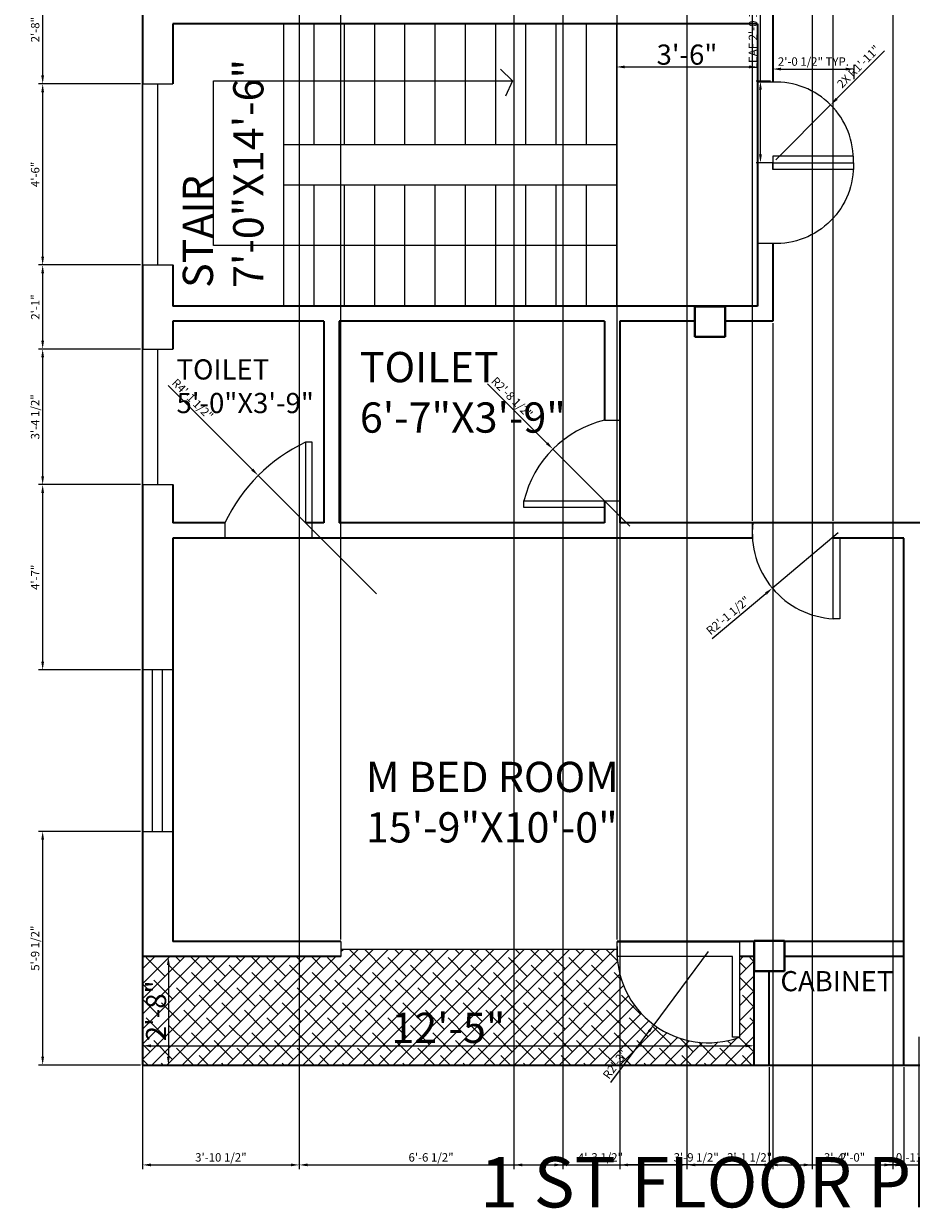
# Model space of a CAD drawing. Units: millimetres. Extents: x 2124 to 2653, y 1244 to 1836.
# Tile 1 of 4: x 2124 to 2389, y 1244 to 1597. Entities that reach past the tile are written whole.
import ezdxf

# ---------------------------------------------------------------- set-up
doc = ezdxf.new("R2010")
doc.units = ezdxf.units.MM
for name, color, linetype, lineweight in [('A-ANNO-DIMS', 2, 'Continuous', 18), ('A-ANNO-TEXT', 7, 'Continuous', 18), ('A-ANNO-TITL', 7, 'Continuous', 35), ('A-AREA-IDEN', 7, 'Continuous', 18), ('A-COLS', 1, 'Continuous', 40), ('A-DOOR', 3, 'Continuous', 18), ('A-FLOR-PATT', 252, 'Continuous', 13), ('A-FLOR-STRS', 32, 'Continuous', 18), ('A-GLAZ', 4, 'Continuous', 18), ('A-WALL', 7, 'Continuous', 35)]:
    doc.layers.add(name, color=color, linetype=linetype, lineweight=lineweight)
doc.styles.get("Standard").update_dxf_attribs({"font": 'arial.ttf'})
doc.dimstyles.new('ISO-25', dxfattribs={"dimtxt": 2.5, "dimasz": 2.5, "dimexe": 1.25, "dimexo": 0.625, "dimtad": 1, "dimdec": 0, "dimlunit": 3, "dimtxsty": 'Standard', "dimcen": 2.5, "dimadec": 0, "dimazin": 0, "dimtfac": 1, "dimtdec": 0, "dimtmove": 0, "dimatfit": 3, "dimfxl": 1, "dimarcsym": 0})

# ---------------------------------------------------------------- blocks, each defined once
blk = doc.blocks.new('*D1')
at = {"layer": 'A-ANNO-DIMS', "color": 0, "lineweight": -2, "transparency": 16777216}
for p, q in [((2300.76, 1596.12), (2300.76, 1582.64)), ((2342.76, 1596.12), (2342.76, 1582.64)), ((2303.26, 1583.89), (2340.26, 1583.89))]:
    blk.add_line(p, q, dxfattribs=at)
at = {"layer": 'A-ANNO-DIMS', "color": 0, "transparency": 16777216}
for points in [[(2303.26, 1584.31), (2303.26, 1583.47), (2300.76, 1583.89)], [(2340.26, 1584.31), (2340.26, 1583.47), (2342.76, 1583.89)]]:
    blk.add_solid(points, dxfattribs=at)
at = {"layer": 'Defpoints', "color": 0, "transparency": 16777216}
for p in [(2300.76, 1596.74), (2342.76, 1596.74), (2342.76, 1583.89)]:
    blk.add_point(p, dxfattribs=at)
at = {"layer": 'A-ANNO-DIMS', "color": 0, "transparency": 16777216, "insert": (2321.76, 1587.55), "char_height": 2.5, "width": 10.4079, "attachment_point": 5}
blk.add_mtext('{\\fCambria|b0|i0|c0|p18;\\H2.4x;3\'-6"}', dxfattribs=at)
blk = doc.blocks.new('*D5')
at = {"layer": 'A-ANNO-DIMS', "color": 0, "lineweight": -2, "transparency": 16777216}
for p, q in [((2160.38, 1319.24), (2168.7, 1319.24)), ((2167.45, 1316.74), (2167.45, 1289.47)), ((2160.38, 1286.97), (2168.7, 1286.97))]:
    blk.add_line(p, q, dxfattribs=at)
at = {"layer": 'A-ANNO-DIMS', "color": 0, "transparency": 16777216}
for points in [[(2167.04, 1316.74), (2167.87, 1316.74), (2167.45, 1319.24)], [(2167.04, 1289.47), (2167.87, 1289.47), (2167.45, 1286.97)]]:
    blk.add_solid(points, dxfattribs=at)
at = {"layer": 'Defpoints', "color": 0, "transparency": 16777216}
for p in [(2159.76, 1319.24), (2159.76, 1286.97), (2167.45, 1286.97)]:
    blk.add_point(p, dxfattribs=at)
at = {"layer": 'A-ANNO-DIMS', "color": 0, "transparency": 16777216, "insert": (2163.79, 1303.11), "char_height": 2.5, "attachment_point": 5, "rotation": 90}
blk.add_mtext('{\\fCambria|b0|i0|c0|p18;\\H2.4x;2\'-8"}', dxfattribs=at)
blk = doc.blocks.new('*D6')
at = {"layer": 'A-ANNO-DIMS', "color": 0, "lineweight": -2, "transparency": 16777216}
for p, q in [((2159.76, 1287.6), (2159.76, 1293.95)), ((2341.76, 1287.6), (2341.76, 1293.95)), ((2162.26, 1292.7), (2339.26, 1292.7))]:
    blk.add_line(p, q, dxfattribs=at)
at = {"layer": 'A-ANNO-DIMS', "color": 0, "transparency": 16777216}
for points in [[(2162.26, 1293.12), (2162.26, 1292.28), (2159.76, 1292.7)], [(2339.26, 1293.12), (2339.26, 1292.28), (2341.76, 1292.7)]]:
    blk.add_solid(points, dxfattribs=at)
at = {"layer": 'Defpoints', "color": 0, "transparency": 16777216}
for p in [(2341.76, 1292.7), (2159.76, 1286.97), (2341.76, 1286.97)]:
    blk.add_point(p, dxfattribs=at)
at = {"layer": 'A-ANNO-DIMS', "color": 0, "transparency": 16777216, "insert": (2250.76, 1298.04), "char_height": 2.5, "width": 30.6159, "attachment_point": 5}
blk.add_mtext('{\\fCambria|b0|i0|c0|p18;\\H3.6x;12\'-5"}', dxfattribs=at)
blk = doc.blocks.new('WINDOW-4FT')
for p, q in [((48, 9), (0, 9)), ((0, 9), (0, 0)), ((48, 0), (48, 9)), ((48, 6), (0, 6)), ((48, 3), (0, 3)), ((0, 0), (48, 0))]:
    blk.add_line(p, q)
blk = doc.blocks.new('COLUMN-9IN-SQ')
for p, q in [((9, 9), (0, 9)), ((0, 9), (0, 0)), ((9, 0), (9, 9)), ((0, 0), (9, 0))]:
    blk.add_line(p, q)
blk = doc.blocks.new('DOOR-2FT-STAIR-LEAF')
for p, q in [((0, 2), (0, 0)), ((24, 2), (0, 2)), ((24, 0), (24, 2)), ((0, 0), (24, 0))]:
    blk.add_line(p, q)
blk.add_arc((0.91, 0.91), 23.11, 357.7485, 92.2515)
blk = doc.blocks.new('*D20')
at = {"layer": 'A-ANNO-DIMS', "color": 0, "lineweight": -2, "transparency": 16777216}
for p, q in [((2343.62, 1579.62), (2343.62, 1614.03)), ((2346.63, 1579.62), (2342.37, 1579.62)), ((2343.62, 1557.86), (2343.62, 1577.12)), ((2346.63, 1555.36), (2342.37, 1555.36))]:
    blk.add_line(p, q, dxfattribs=at)
at = {"layer": 'A-ANNO-DIMS', "color": 0, "transparency": 16777216}
for points in [[(2343.2, 1577.12), (2344.04, 1577.12), (2343.62, 1579.62)], [(2343.2, 1557.86), (2344.04, 1557.86), (2343.62, 1555.36)]]:
    blk.add_solid(points, dxfattribs=at)
at = {"layer": 'Defpoints', "color": 0, "transparency": 16777216}
for p in [(2343.62, 1579.62), (2347.26, 1579.62), (2347.26, 1555.36)]:
    blk.add_point(p, dxfattribs=at)
at = {"layer": 'A-ANNO-DIMS', "color": 0, "transparency": 16777216, "insert": (2341.7, 1598.07), "char_height": 2.5, "attachment_point": 5, "rotation": 90}
blk.add_mtext('LEAF 2\'-0 1/2" TYP.', dxfattribs=at)
blk = doc.blocks.new('*D21')
at = {"layer": 'A-ANNO-DIMS', "color": 0, "lineweight": -2, "transparency": 16777216}
for p, q in [((2347.26, 1580.24), (2347.26, 1584.51)), ((2349.76, 1583.26), (2369.01, 1583.26)), ((2371.51, 1580.24), (2371.51, 1584.51))]:
    blk.add_line(p, q, dxfattribs=at)
at = {"layer": 'A-ANNO-DIMS', "color": 0, "transparency": 16777216}
for points in [[(2349.76, 1583.67), (2349.76, 1582.84), (2347.26, 1583.26)], [(2369.01, 1583.67), (2369.01, 1582.84), (2371.51, 1583.26)]]:
    blk.add_solid(points, dxfattribs=at)
at = {"layer": 'Defpoints', "color": 0, "transparency": 16777216}
for p in [(2371.51, 1583.26), (2347.26, 1579.62), (2371.51, 1579.62)]:
    blk.add_point(p, dxfattribs=at)
at = {"layer": 'A-ANNO-DIMS', "color": 0, "transparency": 16777216, "insert": (2359.38, 1585.17), "char_height": 2.5, "attachment_point": 5}
blk.add_mtext('2\'-0 1/2" TYP.', dxfattribs=at)
blk = doc.blocks.new('*D29')
at = {"layer": 'A-ANNO-DIMS', "color": 0, "lineweight": -2, "transparency": 16777216}
for p, q in [((2159.13, 1356.5), (2128.81, 1356.5)), ((2130.06, 1289.47), (2130.06, 1354)), ((2159.13, 1286.97), (2128.81, 1286.97))]:
    blk.add_line(p, q, dxfattribs=at)
at = {"layer": 'A-ANNO-DIMS', "color": 0, "transparency": 16777216}
for points in [[(2129.64, 1354), (2130.47, 1354), (2130.06, 1356.5)], [(2129.64, 1289.47), (2130.47, 1289.47), (2130.06, 1286.97)]]:
    blk.add_solid(points, dxfattribs=at)
at = {"layer": 'Defpoints', "color": 0, "transparency": 16777216}
for p in [(2130.06, 1356.5), (2159.76, 1356.5), (2159.76, 1286.97)]:
    blk.add_point(p, dxfattribs=at)
at = {"layer": 'A-ANNO-DIMS', "color": 0, "transparency": 16777216, "insert": (2128.14, 1321.74), "char_height": 2.5, "attachment_point": 5, "rotation": 90}
blk.add_mtext('5\'-9 1/2"', dxfattribs=at)
blk = doc.blocks.new('*D30')
at = {"layer": 'A-ANNO-DIMS', "color": 0, "lineweight": -2, "transparency": 16777216}
for p, q in [((2159.13, 1459.63), (2128.81, 1459.63)), ((2130.06, 1407), (2130.06, 1457.13)), ((2159.13, 1404.5), (2128.81, 1404.5))]:
    blk.add_line(p, q, dxfattribs=at)
at = {"layer": 'A-ANNO-DIMS', "color": 0, "transparency": 16777216}
for points in [[(2129.64, 1457.13), (2130.47, 1457.13), (2130.06, 1459.63)], [(2129.64, 1407), (2130.47, 1407), (2130.06, 1404.5)]]:
    blk.add_solid(points, dxfattribs=at)
at = {"layer": 'Defpoints', "color": 0, "transparency": 16777216}
for p in [(2130.06, 1459.63), (2159.76, 1459.63), (2159.76, 1404.5)]:
    blk.add_point(p, dxfattribs=at)
at = {"layer": 'A-ANNO-DIMS', "color": 0, "transparency": 16777216, "insert": (2128.18, 1432.07), "char_height": 2.5, "attachment_point": 5, "rotation": 90}
blk.add_mtext('4\'-7"', dxfattribs=at)
blk = doc.blocks.new('*D31')
at = {"layer": 'A-ANNO-DIMS', "color": 0, "lineweight": -2, "transparency": 16777216}
for p, q in [((2159.13, 1499.97), (2128.81, 1499.97)), ((2130.06, 1462.13), (2130.06, 1497.47)), ((2159.13, 1459.63), (2128.81, 1459.63))]:
    blk.add_line(p, q, dxfattribs=at)
at = {"layer": 'A-ANNO-DIMS', "color": 0, "transparency": 16777216}
for points in [[(2129.64, 1497.47), (2130.47, 1497.47), (2130.06, 1499.97)], [(2129.64, 1462.13), (2130.47, 1462.13), (2130.06, 1459.63)]]:
    blk.add_solid(points, dxfattribs=at)
at = {"layer": 'Defpoints', "color": 0, "transparency": 16777216}
for p in [(2130.06, 1499.97), (2159.76, 1499.97), (2159.76, 1459.63)]:
    blk.add_point(p, dxfattribs=at)
at = {"layer": 'A-ANNO-DIMS', "color": 0, "transparency": 16777216, "insert": (2128.14, 1479.8), "char_height": 2.5, "attachment_point": 5, "rotation": 90}
blk.add_mtext('3\'-4 1/2"', dxfattribs=at)
blk = doc.blocks.new('*D32')
at = {"layer": 'A-ANNO-DIMS', "color": 0, "lineweight": -2, "transparency": 16777216}
for p, q in [((2159.13, 1524.98), (2128.81, 1524.98)), ((2130.06, 1502.47), (2130.06, 1522.48)), ((2159.13, 1499.97), (2128.81, 1499.97))]:
    blk.add_line(p, q, dxfattribs=at)
at = {"layer": 'A-ANNO-DIMS', "color": 0, "transparency": 16777216}
for points in [[(2129.64, 1522.48), (2130.47, 1522.48), (2130.06, 1524.98)], [(2129.64, 1502.47), (2130.47, 1502.47), (2130.06, 1499.97)]]:
    blk.add_solid(points, dxfattribs=at)
at = {"layer": 'Defpoints', "color": 0, "transparency": 16777216}
for p in [(2130.06, 1524.98), (2159.76, 1524.98), (2159.76, 1499.97)]:
    blk.add_point(p, dxfattribs=at)
at = {"layer": 'A-ANNO-DIMS', "color": 0, "transparency": 16777216, "insert": (2128.18, 1512.47), "char_height": 2.5, "attachment_point": 5, "rotation": 90}
blk.add_mtext('2\'-1"', dxfattribs=at)
blk = doc.blocks.new('*D33')
at = {"layer": 'A-ANNO-DIMS', "color": 0, "lineweight": -2, "transparency": 16777216}
for p, q in [((2159.13, 1578.86), (2128.81, 1578.86)), ((2130.06, 1527.48), (2130.06, 1576.36)), ((2159.13, 1524.98), (2128.81, 1524.98))]:
    blk.add_line(p, q, dxfattribs=at)
at = {"layer": 'A-ANNO-DIMS', "color": 0, "transparency": 16777216}
for points in [[(2129.64, 1576.36), (2130.47, 1576.36), (2130.06, 1578.86)], [(2129.64, 1527.48), (2130.47, 1527.48), (2130.06, 1524.98)]]:
    blk.add_solid(points, dxfattribs=at)
at = {"layer": 'Defpoints', "color": 0, "transparency": 16777216}
for p in [(2130.06, 1578.86), (2159.76, 1578.86), (2159.76, 1524.98)]:
    blk.add_point(p, dxfattribs=at)
at = {"layer": 'A-ANNO-DIMS', "color": 0, "transparency": 16777216, "insert": (2128.15, 1551.92), "char_height": 2.5, "attachment_point": 5, "rotation": 90}
blk.add_mtext('4\'-6"', dxfattribs=at)
blk = doc.blocks.new('*D34')
at = {"layer": 'A-ANNO-DIMS', "color": 0, "lineweight": -2, "transparency": 16777216}
for p, q in [((2159.13, 1611.09), (2128.81, 1611.09)), ((2130.06, 1581.36), (2130.06, 1608.59)), ((2159.13, 1578.86), (2128.81, 1578.86))]:
    blk.add_line(p, q, dxfattribs=at)
at = {"layer": 'A-ANNO-DIMS', "color": 0, "transparency": 16777216}
for points in [[(2129.64, 1608.59), (2130.47, 1608.59), (2130.06, 1611.09)], [(2129.64, 1581.36), (2130.47, 1581.36), (2130.06, 1578.86)]]:
    blk.add_solid(points, dxfattribs=at)
at = {"layer": 'Defpoints', "color": 0, "transparency": 16777216}
for p in [(2130.06, 1611.09), (2159.76, 1611.09), (2159.76, 1578.86)]:
    blk.add_point(p, dxfattribs=at)
at = {"layer": 'A-ANNO-DIMS', "color": 0, "transparency": 16777216, "insert": (2128.15, 1594.98), "char_height": 2.5, "attachment_point": 5, "rotation": 90}
blk.add_mtext('2\'-8"', dxfattribs=at)
blk = doc.blocks.new('*D36')
at = {"layer": 'A-ANNO-DIMS', "color": 0, "lineweight": -2, "transparency": 16777216}
for p, q in [((2159.76, 1753.12), (2159.76, 1256.02)), ((2206.41, 1748.62), (2206.41, 1256.02)), ((2162.26, 1257.27), (2203.91, 1257.27))]:
    blk.add_line(p, q, dxfattribs=at)
at = {"layer": 'A-ANNO-DIMS', "color": 0, "transparency": 16777216}
for points in [[(2162.26, 1257.69), (2162.26, 1256.86), (2159.76, 1257.27)], [(2203.91, 1257.69), (2203.91, 1256.86), (2206.41, 1257.27)]]:
    blk.add_solid(points, dxfattribs=at)
at = {"layer": 'Defpoints', "color": 0, "transparency": 16777216}
for p in [(2159.76, 1753.74), (2206.41, 1749.24), (2206.41, 1257.27)]:
    blk.add_point(p, dxfattribs=at)
at = {"layer": 'A-ANNO-DIMS', "color": 0, "transparency": 16777216, "insert": (2183.08, 1259.19), "char_height": 2.5, "attachment_point": 5}
blk.add_mtext('3\'-10 1/2"', dxfattribs=at)
blk = doc.blocks.new('*D37')
at = {"layer": 'A-ANNO-DIMS', "color": 0, "lineweight": -2, "transparency": 16777216}
for p, q in [((2206.41, 1748.62), (2206.41, 1256.02)), ((2284.8, 1748.62), (2284.8, 1256.02)), ((2208.91, 1257.27), (2282.3, 1257.27))]:
    blk.add_line(p, q, dxfattribs=at)
at = {"layer": 'A-ANNO-DIMS', "color": 0, "transparency": 16777216}
for points in [[(2208.91, 1257.69), (2208.91, 1256.86), (2206.41, 1257.27)], [(2282.3, 1257.69), (2282.3, 1256.86), (2284.8, 1257.27)]]:
    blk.add_solid(points, dxfattribs=at)
at = {"layer": 'Defpoints', "color": 0, "transparency": 16777216}
for p in [(2206.41, 1749.24), (2284.8, 1749.24), (2284.8, 1257.27)]:
    blk.add_point(p, dxfattribs=at)
at = {"layer": 'A-ANNO-DIMS', "color": 0, "transparency": 16777216, "insert": (2245.61, 1259.19), "char_height": 2.5, "attachment_point": 5}
blk.add_mtext('6\'-6 1/2"', dxfattribs=at)
blk = doc.blocks.new('*D38')
at = {"layer": 'A-ANNO-DIMS', "color": 0, "lineweight": -2, "transparency": 16777216}
for p, q in [((2159.76, 1319.87), (2159.76, 1814.69)), ((2162.26, 1813.44), (2216.31, 1813.44)), ((2218.81, 1324.37), (2218.81, 1814.69))]:
    blk.add_line(p, q, dxfattribs=at)
at = {"layer": 'A-ANNO-DIMS', "color": 0, "transparency": 16777216}
for points in [[(2162.26, 1813.86), (2162.26, 1813.02), (2159.76, 1813.44)], [(2216.31, 1813.86), (2216.31, 1813.02), (2218.81, 1813.44)]]:
    blk.add_solid(points, dxfattribs=at)
at = {"layer": 'Defpoints', "color": 0, "transparency": 16777216}
for p in [(2218.81, 1813.44), (2218.81, 1323.74), (2159.76, 1319.24)]:
    blk.add_point(p, dxfattribs=at)
at = {"layer": 'A-ANNO-DIMS', "color": 0, "transparency": 16777216, "insert": (2189.28, 1815.32), "char_height": 2.5, "attachment_point": 5}
blk.add_mtext('4\'-11"', dxfattribs=at)
blk = doc.blocks.new('*D39')
at = {"layer": 'A-ANNO-DIMS', "color": 0, "lineweight": -2, "transparency": 16777216}
for p, q in [((2218.81, 1324.37), (2218.81, 1814.69)), ((2221.31, 1813.44), (2298.49, 1813.44)), ((2300.99, 1324.37), (2300.99, 1814.69))]:
    blk.add_line(p, q, dxfattribs=at)
at = {"layer": 'A-ANNO-DIMS', "color": 0, "transparency": 16777216}
for points in [[(2221.31, 1813.86), (2221.31, 1813.02), (2218.81, 1813.44)], [(2298.49, 1813.86), (2298.49, 1813.02), (2300.99, 1813.44)]]:
    blk.add_solid(points, dxfattribs=at)
at = {"layer": 'Defpoints', "color": 0, "transparency": 16777216}
for p in [(2300.99, 1813.44), (2218.81, 1323.74), (2300.99, 1323.74)]:
    blk.add_point(p, dxfattribs=at)
at = {"layer": 'A-ANNO-DIMS', "color": 0, "transparency": 16777216, "insert": (2259.9, 1815.34), "char_height": 2.5, "attachment_point": 5}
blk.add_mtext('6\'-10"', dxfattribs=at)
blk = doc.blocks.new('*D40')
at = {"layer": 'A-ANNO-DIMS', "color": 0, "lineweight": -2, "transparency": 16777216}
for p, q in [((2270.27, 1645.62), (2270.27, 1256.02)), ((2321.76, 1645.62), (2321.76, 1256.02)), ((2272.77, 1257.27), (2319.26, 1257.27))]:
    blk.add_line(p, q, dxfattribs=at)
at = {"layer": 'A-ANNO-DIMS', "color": 0, "transparency": 16777216}
for points in [[(2272.77, 1257.69), (2272.77, 1256.86), (2270.27, 1257.27)], [(2319.26, 1257.69), (2319.26, 1256.86), (2321.76, 1257.27)]]:
    blk.add_solid(points, dxfattribs=at)
at = {"layer": 'Defpoints', "color": 0, "transparency": 16777216}
for p in [(2270.27, 1646.24), (2321.76, 1646.24), (2321.76, 1257.27)]:
    blk.add_point(p, dxfattribs=at)
at = {"layer": 'A-ANNO-DIMS', "color": 0, "transparency": 16777216, "insert": (2296.01, 1259.19), "char_height": 2.5, "attachment_point": 5}
blk.add_mtext('4\'-3 1/2"', dxfattribs=at)
blk = doc.blocks.new('*D41')
at = {"layer": 'A-ANNO-DIMS', "color": 0, "lineweight": -2, "transparency": 16777216}
for p, q in [((2321.76, 1645.62), (2321.76, 1256.02)), ((2359.02, 1645.62), (2359.02, 1256.02)), ((2324.26, 1257.27), (2356.52, 1257.27))]:
    blk.add_line(p, q, dxfattribs=at)
at = {"layer": 'A-ANNO-DIMS', "color": 0, "transparency": 16777216}
for points in [[(2324.26, 1257.69), (2324.26, 1256.86), (2321.76, 1257.27)], [(2356.52, 1257.69), (2356.52, 1256.86), (2359.02, 1257.27)]]:
    blk.add_solid(points, dxfattribs=at)
at = {"layer": 'Defpoints', "color": 0, "transparency": 16777216}
for p in [(2321.76, 1646.24), (2359.02, 1646.24), (2359.02, 1257.27)]:
    blk.add_point(p, dxfattribs=at)
at = {"layer": 'A-ANNO-DIMS', "color": 0, "transparency": 16777216, "insert": (2340.39, 1259.19), "char_height": 2.5, "attachment_point": 5}
blk.add_mtext('3\'-1 1/2"', dxfattribs=at)
blk = doc.blocks.new('*D42')
at = {"layer": 'A-ANNO-DIMS', "color": 0, "lineweight": -2, "transparency": 16777216}
for p, q in [((2359.02, 1645.62), (2359.02, 1256.02)), ((2383.02, 1645.62), (2383.02, 1256.02)), ((2361.52, 1257.27), (2380.52, 1257.27))]:
    blk.add_line(p, q, dxfattribs=at)
at = {"layer": 'A-ANNO-DIMS', "color": 0, "transparency": 16777216}
for points in [[(2361.52, 1257.69), (2361.52, 1256.86), (2359.02, 1257.27)], [(2380.52, 1257.69), (2380.52, 1256.86), (2383.02, 1257.27)]]:
    blk.add_solid(points, dxfattribs=at)
at = {"layer": 'Defpoints', "color": 0, "transparency": 16777216}
for p in [(2359.02, 1646.24), (2383.02, 1646.24), (2383.02, 1257.27)]:
    blk.add_point(p, dxfattribs=at)
at = {"layer": 'A-ANNO-DIMS', "color": 0, "transparency": 16777216, "insert": (2371.02, 1259.18), "char_height": 2.5, "attachment_point": 5}
blk.add_mtext('2\'-0"', dxfattribs=at)
blk = doc.blocks.new('*D43')
at = {"layer": 'A-ANNO-DIMS', "color": 0, "lineweight": -2, "transparency": 16777216}
for p, q in [((2383.02, 1645.62), (2383.02, 1256.02)), ((2394.21, 1645.62), (2394.21, 1256.02)), ((2385.52, 1257.27), (2391.71, 1257.27))]:
    blk.add_line(p, q, dxfattribs=at)
at = {"layer": 'A-ANNO-DIMS', "color": 0, "transparency": 16777216}
for points in [[(2385.52, 1257.69), (2385.52, 1256.86), (2383.02, 1257.27)], [(2391.71, 1257.69), (2391.71, 1256.86), (2394.21, 1257.27)]]:
    blk.add_solid(points, dxfattribs=at)
at = {"layer": 'Defpoints', "color": 0, "transparency": 16777216}
for p in [(2383.02, 1646.24), (2394.21, 1646.24), (2394.21, 1257.27)]:
    blk.add_point(p, dxfattribs=at)
at = {"layer": 'A-ANNO-DIMS', "color": 0, "transparency": 16777216, "insert": (2388.62, 1259.18), "char_height": 2.5, "attachment_point": 5}
blk.add_mtext('0\'-11"', dxfattribs=at)
blk = doc.blocks.new('*D46')
at = {"layer": 'A-ANNO-DIMS', "color": 0, "lineweight": -2, "transparency": 16777216}
for p, q in [((2341.24, 1448.87), (2341.24, 1814.69)), ((2343.74, 1813.44), (2362.74, 1813.44)), ((2365.24, 1448.87), (2365.24, 1814.69))]:
    blk.add_line(p, q, dxfattribs=at)
at = {"layer": 'A-ANNO-DIMS', "color": 0, "transparency": 16777216}
for points in [[(2343.74, 1813.86), (2343.74, 1813.02), (2341.24, 1813.44)], [(2362.74, 1813.86), (2362.74, 1813.02), (2365.24, 1813.44)]]:
    blk.add_solid(points, dxfattribs=at)
at = {"layer": 'Defpoints', "color": 0, "transparency": 16777216}
for p in [(2365.24, 1813.44), (2341.24, 1448.24), (2365.24, 1448.24)]:
    blk.add_point(p, dxfattribs=at)
at = {"layer": 'A-ANNO-DIMS', "color": 0, "transparency": 16777216, "insert": (2353.24, 1815.34), "char_height": 2.5, "attachment_point": 5}
blk.add_mtext('2\'-0"', dxfattribs=at)
blk = doc.blocks.new('*D47')
at = {"layer": 'A-ANNO-DIMS', "color": 0, "lineweight": -2, "transparency": 16777216}
for p, q in [((2365.24, 1448.87), (2365.24, 1814.69)), ((2367.74, 1813.44), (2394.29, 1813.44)), ((2396.79, 1448.87), (2396.79, 1814.69))]:
    blk.add_line(p, q, dxfattribs=at)
at = {"layer": 'A-ANNO-DIMS', "color": 0, "transparency": 16777216}
for points in [[(2367.74, 1813.86), (2367.74, 1813.02), (2365.24, 1813.44)], [(2394.29, 1813.86), (2394.29, 1813.02), (2396.79, 1813.44)]]:
    blk.add_solid(points, dxfattribs=at)
at = {"layer": 'Defpoints', "color": 0, "transparency": 16777216}
for p in [(2396.79, 1813.44), (2365.24, 1448.24), (2396.79, 1448.24)]:
    blk.add_point(p, dxfattribs=at)
at = {"layer": 'A-ANNO-DIMS', "color": 0, "transparency": 16777216, "insert": (2381.02, 1815.36), "char_height": 2.5, "attachment_point": 5}
blk.add_mtext('2\'-7 1/2"', dxfattribs=at)
blk = doc.blocks.new('*D50')
at = {"layer": 'A-ANNO-DIMS', "color": 0, "lineweight": -2, "transparency": 16777216}
for p, q in [((2301.76, 1507.62), (2301.76, 1256.02)), ((2347.26, 1507.62), (2347.26, 1256.02)), ((2344.76, 1257.27), (2304.26, 1257.27))]:
    blk.add_line(p, q, dxfattribs=at)
at = {"layer": 'A-ANNO-DIMS', "color": 0, "transparency": 16777216}
for points in [[(2304.26, 1257.69), (2304.26, 1256.86), (2301.76, 1257.27)], [(2344.76, 1257.69), (2344.76, 1256.86), (2347.26, 1257.27)]]:
    blk.add_solid(points, dxfattribs=at)
at = {"layer": 'Defpoints', "color": 0, "transparency": 16777216}
for p in [(2301.76, 1508.24), (2347.26, 1508.24), (2301.76, 1257.27)]:
    blk.add_point(p, dxfattribs=at)
at = {"layer": 'A-ANNO-DIMS', "color": 0, "transparency": 16777216, "insert": (2324.51, 1259.19), "char_height": 2.5, "attachment_point": 5}
blk.add_mtext('3\'-9 1/2"', dxfattribs=at)
blk = doc.blocks.new('*D51')
at = {"layer": 'A-ANNO-DIMS', "color": 0, "lineweight": -2, "transparency": 16777216}
for p, q in [((2346.26, 1286.35), (2346.26, 1256.02)), ((2386.26, 1286.35), (2386.26, 1256.02)), ((2348.76, 1257.27), (2383.76, 1257.27))]:
    blk.add_line(p, q, dxfattribs=at)
at = {"layer": 'A-ANNO-DIMS', "color": 0, "transparency": 16777216}
for points in [[(2348.76, 1257.69), (2348.76, 1256.86), (2346.26, 1257.27)], [(2383.76, 1257.69), (2383.76, 1256.86), (2386.26, 1257.27)]]:
    blk.add_solid(points, dxfattribs=at)
at = {"layer": 'Defpoints', "color": 0, "transparency": 16777216}
for p in [(2346.26, 1286.97), (2386.26, 1286.97), (2386.26, 1257.27)]:
    blk.add_point(p, dxfattribs=at)
at = {"layer": 'A-ANNO-DIMS', "color": 0, "transparency": 16777216, "insert": (2366.26, 1259.18), "char_height": 2.5, "attachment_point": 5}
blk.add_mtext('3\'-4"', dxfattribs=at)
blk = doc.blocks.new('*D52')
at = {"layer": 'A-ANNO-DIMS', "color": 0, "lineweight": -2, "transparency": 16777216}
for p, q in [((2390.76, 1295.35), (2390.76, 1256.02)), ((2386.26, 1286.35), (2386.26, 1256.02)), ((2383.76, 1257.27), (2381.26, 1257.27)), ((2386.26, 1257.27), (2390.76, 1257.27)), ((2393.26, 1257.27), (2409.48, 1257.27))]:
    blk.add_line(p, q, dxfattribs=at)
at = {"layer": 'A-ANNO-DIMS', "color": 0, "transparency": 16777216}
for points in [[(2383.76, 1257.69), (2383.76, 1256.86), (2386.26, 1257.27)], [(2393.26, 1257.69), (2393.26, 1256.86), (2390.76, 1257.27)]]:
    blk.add_solid(points, dxfattribs=at)
at = {"layer": 'Defpoints', "color": 0, "transparency": 16777216}
for p in [(2390.76, 1295.97), (2386.26, 1286.97), (2390.76, 1257.27)]:
    blk.add_point(p, dxfattribs=at)
at = {"layer": 'A-ANNO-DIMS', "color": 0, "transparency": 16777216, "insert": (2402.62, 1259.19), "char_height": 2.5, "attachment_point": 5}
blk.add_mtext('0\'-4 1/2"', dxfattribs=at)
blk = doc.blocks.new('*D53')
at = {"layer": 'A-ANNO-DIMS', "color": 0, "lineweight": -2, "transparency": 16777216}
for p, q in [((2167.39, 1489.14), (2192.41, 1464.12)), ((2229.34, 1427.2), (2194.18, 1462.35))]:
    blk.add_line(p, q, dxfattribs=at)
at = {"layer": 'A-ANNO-DIMS', "color": 0, "transparency": 16777216}
blk.add_solid([(2192.71, 1464.41), (2192.12, 1463.83), (2194.18, 1462.35)], dxfattribs=at)
at = {"layer": 'Defpoints', "color": 0, "transparency": 16777216}
for p in [(2194.18, 1462.35), (2229.34, 1427.2)]:
    blk.add_point(p, dxfattribs=at)
at = {"layer": 'A-ANNO-DIMS', "color": 0, "transparency": 16777216, "insert": (2174.44, 1484.8), "char_height": 2.5, "attachment_point": 5, "rotation": 315.0002}
blk.add_mtext('R4\'-1 1/2"', dxfattribs=at)
blk = doc.blocks.new('*D57')
at = {"layer": 'A-ANNO-DIMS', "color": 0, "lineweight": -2, "transparency": 16777216}
for p, q in [((2262.41, 1489.67), (2280.1, 1471.98)), ((2304.8, 1447.28), (2281.87, 1470.21))]:
    blk.add_line(p, q, dxfattribs=at)
at = {"layer": 'A-ANNO-DIMS', "color": 0, "transparency": 16777216}
blk.add_solid([(2280.39, 1472.27), (2279.8, 1471.69), (2281.87, 1470.21)], dxfattribs=at)
at = {"layer": 'Defpoints', "color": 0, "transparency": 16777216}
for p in [(2281.87, 1470.21), (2304.8, 1447.28)]:
    blk.add_point(p, dxfattribs=at)
at = {"layer": 'A-ANNO-DIMS', "color": 0, "transparency": 16777216, "insert": (2269.46, 1485.33), "char_height": 2.5, "attachment_point": 5, "rotation": 314.9995}
blk.add_mtext('R2\'-8 1/2"', dxfattribs=at)
blk = doc.blocks.new('*D59')
at = {"layer": 'A-ANNO-DIMS', "color": 0, "lineweight": -2, "transparency": 16777216}
for p, q in [((2328.07, 1320.74), (2311.9, 1298.95)), ((2299.13, 1281.75), (2310.41, 1296.95))]:
    blk.add_line(p, q, dxfattribs=at)
at = {"layer": 'A-ANNO-DIMS', "color": 0, "transparency": 16777216}
blk.add_solid([(2310.08, 1297.2), (2310.75, 1296.7), (2311.9, 1298.95)], dxfattribs=at)
at = {"layer": 'Defpoints', "color": 0, "transparency": 16777216}
for p in [(2328.07, 1320.74), (2311.9, 1298.95)]:
    blk.add_point(p, dxfattribs=at)
at = {"layer": 'A-ANNO-DIMS', "color": 0, "transparency": 16777216, "insert": (2300.67, 1287.02), "char_height": 2.5, "attachment_point": 5, "rotation": 53.4104}
blk.add_mtext('R2\'-3"', dxfattribs=at)
blk = doc.blocks.new('*D60')
at = {"layer": 'A-ANNO-DIMS', "color": 0, "lineweight": -2, "transparency": 16777216}
for p, q in [((2366.77, 1445.27), (2347.17, 1428.85)), ((2329.23, 1413.82), (2345.25, 1427.24))]:
    blk.add_line(p, q, dxfattribs=at)
at = {"layer": 'A-ANNO-DIMS', "color": 0, "transparency": 16777216}
blk.add_solid([(2344.98, 1427.56), (2345.52, 1426.92), (2347.17, 1428.85)], dxfattribs=at)
at = {"layer": 'Defpoints', "color": 0, "transparency": 16777216}
for p in [(2366.77, 1445.27), (2347.17, 1428.85)]:
    blk.add_point(p, dxfattribs=at)
at = {"layer": 'A-ANNO-DIMS', "color": 0, "transparency": 16777216, "insert": (2334.17, 1420.46), "char_height": 2.5, "attachment_point": 5, "rotation": 39.9512}
blk.add_mtext('R2\'-1 1/2"', dxfattribs=at)
blk = doc.blocks.new('*D62')
at = {"layer": 'A-ANNO-DIMS', "color": 0, "lineweight": -2, "transparency": 16777216}
for p, q in [((2380.55, 1588.66), (2366.27, 1574.38)), ((2348.16, 1556.27), (2364.51, 1572.61))]:
    blk.add_line(p, q, dxfattribs=at)
at = {"layer": 'A-ANNO-DIMS', "color": 0, "transparency": 16777216}
blk.add_solid([(2365.98, 1574.68), (2366.57, 1574.09), (2364.51, 1572.61)], dxfattribs=at)
at = {"layer": 'Defpoints', "color": 0, "transparency": 16777216}
for p in [(2364.51, 1572.61), (2348.16, 1556.27)]:
    blk.add_point(p, dxfattribs=at)
at = {"layer": 'A-ANNO-DIMS', "color": 0, "transparency": 16777216, "insert": (2372.98, 1583.75), "char_height": 2.5, "attachment_point": 5, "rotation": 45.0009}
blk.add_mtext('2X R1\'-11"', dxfattribs=at)

msp = doc.modelspace()

# ---------------------------------------------------------------- hatches: boundary and pattern name
at = {"layer": 'A-FLOR-PATT'}
h = msp.add_hatch(dxfattribs=at)
h.set_pattern_fill('ANSI38', color=256)
h.paths.add_polyline_path([(2321.76, 1783.74), (2159.76, 1783.74), (2159.76, 1753.74), (2206.41, 1753.74), (2206.41, 1751.49), (2284.8, 1751.49), (2284.8, 1753.74), (2321.76, 1753.74)])
h.paths.add_polyline_path([(2300.96, 1321.49), (2218.81, 1321.49), (2218.81, 1319.24), (2159.76, 1319.24), (2159.76, 1286.97), (2341.76, 1286.97), (2341.76, 1319.24), (2337.34, 1319.24), (2337.34, 1295.24, -0.529331)])
h.paths.add_polyline_path([(2169.36, 1293.27), (2169.36, 1312.93), (2157.68, 1312.93), (2157.68, 1293.27)], flags=9)
h.paths.add_polyline_path([(2232.46, 1289.84), (2268.72, 1289.84), (2268.72, 1306.74), (2232.46, 1306.74)], flags=24)

# ---------------------------------------------------------------- linework, layer by layer
at = {"layer": 'A-DOOR'}
for p, q in [((2347.26, 1579.36), (2342.76, 1579.36)), ((2347.26, 1555.36), (2342.76, 1555.36)), ((2347.26, 1557.36), (2347.26, 1553.36)), ((2347.26, 1531.36), (2342.76, 1531.36)), ((2297.26, 1478.82), (2301.76, 1478.82)), ((2210.29, 1472.24), (2208.29, 1472.24)), ((2208.29, 1472.24), (2208.29, 1448.24)), ((2210.29, 1448.24), (2210.29, 1472.24)), ((2273.26, 1452.82), (2273.26, 1454.82)), ((2273.26, 1454.82), (2301.76, 1454.82)), ((2297.26, 1452.82), (2273.26, 1452.82)), ((2184.29, 1448.24), (2184.29, 1443.74)), ((2210.29, 1443.74), (2210.29, 1448.24)), ((2341.24, 1443.74), (2341.24, 1448.24)), ((2365.24, 1419.74), (2365.24, 1448.24)), ((2367.24, 1443.74), (2367.24, 1419.74)), ((2367.24, 1419.74), (2365.24, 1419.74)), ((2337.34, 1323.74), (2337.34, 1319.24)), ((2335.34, 1319.24), (2300.99, 1319.24)), ((2335.34, 1295.24), (2335.34, 1319.24)), ((2337.34, 1319.24), (2337.34, 1295.24)), ((2337.34, 1295.24), (2335.34, 1295.24))]:
    msp.add_line(p, q, dxfattribs=at)
for centre, radius, start, end in [((2304.8, 1447.28), 32.43, 103.4517, 166.5483), ((2229.34, 1427.2), 49.72, 115.0414, 154.9586), ((2366.77, 1445.27), 25.58, 173.3333, 266.5689), ((2328.07, 1320.74), 27.13, 176.8409, 289.9798)]:
    msp.add_arc(centre, radius, start, end, dxfattribs=at)
at = {"layer": 'A-FLOR-STRS'}
for p, q in [((2201.76, 1596.74), (2201.76, 1512.74)), ((2210.76, 1596.74), (2210.76, 1560.74)), ((2219.76, 1596.74), (2219.76, 1560.74)), ((2228.76, 1596.74), (2228.76, 1560.74)), ((2237.76, 1596.74), (2237.76, 1560.74)), ((2246.76, 1596.74), (2246.76, 1560.74)), ((2255.76, 1596.74), (2255.76, 1560.74)), ((2264.76, 1596.74), (2264.76, 1560.74)), ((2273.76, 1596.74), (2273.76, 1560.74)), ((2282.76, 1596.74), (2282.76, 1560.74)), ((2291.76, 1596.74), (2291.76, 1560.74)), ((2300.76, 1596.74), (2300.76, 1512.74)), ((2269.81, 1579.73), (2266.24, 1583.23)), ((2180.88, 1530.74), (2180.88, 1579.73)), ((2180.88, 1579.73), (2269.81, 1579.73)), ((2269.81, 1579.73), (2267.78, 1575.16)), ((2300.76, 1560.74), (2201.76, 1560.74)), ((2300.76, 1548.74), (2201.76, 1548.74)), ((2210.76, 1548.74), (2210.76, 1512.74)), ((2219.76, 1548.74), (2219.76, 1512.74)), ((2228.76, 1548.74), (2228.76, 1512.74)), ((2237.76, 1548.74), (2237.76, 1512.74)), ((2246.76, 1548.74), (2246.76, 1512.74)), ((2255.76, 1548.74), (2255.76, 1512.74)), ((2264.76, 1548.74), (2264.76, 1512.74)), ((2273.76, 1548.74), (2273.76, 1512.74)), ((2282.76, 1548.74), (2282.76, 1512.74)), ((2291.76, 1548.74), (2291.76, 1512.74)), ((2210.76, 1530.74), (2180.88, 1530.74)), ((2300.76, 1530.74), (2210.76, 1530.74)), ((2210.76, 1530.74), (2210.76, 1530.74)), ((2300.76, 1530.74), (2300.76, 1512.74))]:
    msp.add_line(p, q, dxfattribs=at)
at = {"layer": 'A-GLAZ'}
for p, q in [((2159.76, 1578.86), (2168.76, 1578.86)), ((2164.26, 1578.86), (2164.26, 1524.98)), ((2159.76, 1524.98), (2168.76, 1524.98)), ((2159.76, 1499.97), (2168.76, 1499.97)), ((2164.26, 1499.97), (2164.26, 1459.63)), ((2159.76, 1459.63), (2168.76, 1459.63)), ((2218.81, 1323.74), (2218.81, 1319.24)), ((2218.81, 1321.49), (2300.99, 1321.49)), ((2300.99, 1319.24), (2300.99, 1323.74))]:
    msp.add_line(p, q, dxfattribs=at)
at = {"layer": 'A-WALL'}
for p, q in [((2159.76, 1611.09), (2159.76, 1578.86)), ((2347.26, 1601.24), (2347.26, 1579.36)), ((2168.76, 1596.74), (2168.76, 1578.86)), ((2342.76, 1596.74), (2168.76, 1596.74)), ((2342.76, 1596.74), (2342.76, 1512.74)), ((2347.26, 1531.36), (2347.26, 1508.24)), ((2159.76, 1524.98), (2159.76, 1499.97)), ((2168.76, 1524.98), (2168.76, 1512.74)), ((2342.76, 1512.74), (2168.76, 1512.74)), ((2213.76, 1508.24), (2168.76, 1508.24)), ((2168.76, 1508.24), (2168.76, 1499.97)), ((2213.76, 1508.24), (2213.76, 1448.24)), ((2218.26, 1508.24), (2218.26, 1448.24)), ((2297.26, 1508.24), (2218.26, 1508.24)), ((2297.26, 1508.24), (2297.26, 1478.82)), ((2301.76, 1508.24), (2301.76, 1448.24)), ((2324.08, 1508.24), (2301.76, 1508.24)), ((2347.26, 1508.24), (2333.08, 1508.24)), ((2159.76, 1459.63), (2159.76, 1286.97)), ((2168.76, 1459.63), (2168.76, 1448.24)), ((2297.26, 1454.82), (2297.26, 1448.24)), ((2184.29, 1448.24), (2168.76, 1448.24)), ((2213.76, 1448.24), (2208.29, 1448.24)), ((2297.26, 1448.24), (2218.26, 1448.24)), ((2534.76, 1448.24), (2301.76, 1448.24)), ((2341.24, 1443.74), (2168.76, 1443.74)), ((2168.76, 1443.74), (2168.76, 1323.74)), ((2386.26, 1443.74), (2365.24, 1443.74)), ((2386.26, 1286.97), (2386.26, 1443.74)), ((2218.81, 1323.74), (2168.76, 1323.74)), ((2300.99, 1323.74), (2337.34, 1323.74)), ((2341.76, 1323.74), (2300.99, 1323.74)), ((2386.26, 1323.74), (2350.76, 1323.74)), ((2218.81, 1319.24), (2159.76, 1319.24)), ((2341.76, 1319.24), (2337.34, 1319.24)), ((2341.76, 1286.97), (2341.76, 1319.24)), ((2386.26, 1319.24), (2350.76, 1319.24)), ((2346.26, 1286.97), (2346.26, 1314.94)), ((2159.76, 1286.97), (2543.76, 1286.97))]:
    msp.add_line(p, q, dxfattribs=at)

# ---------------------------------------------------------------- block references
at = {"layer": 'A-COLS'}
for p in [(2324.08, 1503.61), (2341.76, 1314.94)]:
    msp.add_blockref('COLUMN-9IN-SQ', p, dxfattribs=at)
at = {"layer": 'A-DOOR'}
msp.add_blockref('DOOR-2FT-STAIR-LEAF', (2347.26, 1555.36), dxfattribs=at)
at = {"layer": 'A-DOOR', "extrusion": (0, 0, -1), "zscale": -1, "rotation": 180}
msp.add_blockref('DOOR-2FT-STAIR-LEAF', (-2347.26, 1555.36), dxfattribs=at)
at = {"layer": 'A-GLAZ', "rotation": 270.0000000000007}
msp.add_blockref('WINDOW-4FT', (2159.76, 1404.5), dxfattribs=at)

# ---------------------------------------------------------------- texts
at = {"layer": 'A-ANNO-TEXT', "insert": (2349.56, 1314.94), "char_height": 6, "attachment_point": 1}
msp.add_mtext_dynamic_manual_height_columns('{\\fCambria|b0|i0|c0|p18;CABINET}', width=31.9268, gutter_width=12.5, heights=[0], dxfattribs=at)
at = {"layer": 'A-ANNO-TITL', "insert": (2260.19, 1259.63), "char_height": 15, "attachment_point": 1}
msp.add_mtext_dynamic_manual_height_columns('{\\fCambria|b0|i0|c0|p18;1 ST FLOOR PLAN}', width=375.7159, gutter_width=12.5, heights=[0], dxfattribs=at)
at = {"layer": 'A-AREA-IDEN', "insert": (2171.74, 1518.16), "char_height": 9, "attachment_point": 1, "rotation": 90}
msp.add_mtext_dynamic_manual_height_columns('{\\fCambria|b0|i0|c0|p18;STAIR\\P7\'-0"X14\'-6"}', width=70.2274, gutter_width=12.5, heights=[0], dxfattribs=at)
at = {"layer": 'A-AREA-IDEN', "attachment_point": 1}
for s, width, insert, char_height in [('{\\fCambria|b0|i0|c0|p18;TOILET\\P6\'-7"X3\'-9"}', 49.2648, (2224.43, 1499.1), 9), ('{\\fCambria|b0|i0|c0|p18;TOILET\\P5\'-0"X3\'-9"}', 33.3966, (2169.9, 1496.91), 6), ('{\\fCambria|b0|i0|c0|p18;M BED ROOM\\P15\'-9"X10\'-0"}', 110.4847, (2226.24, 1377.19), 9)]:
    msp.add_mtext_dynamic_manual_height_columns(s, width=width, gutter_width=12.5, heights=[0], dxfattribs=dict(at, insert=insert, char_height=char_height))

# ---------------------------------------------------------------- dimensions: what is measured, and where the dimension line sits
at = {"layer": 'A-ANNO-DIMS'}
for base, p1, p2, picture, middle in [((2396.7929, 1813.4406), (2365.2427, 1448.2406), (2396.7929, 1448.2406), '*D47', (2381.0178, 1815.3582)), ((2218.8056, 1813.4406), (2159.7564, 1319.2406), (2218.8056, 1323.7406), '*D38', (2189.281, 1815.3207)), ((2300.99, 1813.44), (2218.81, 1323.74), (2300.99, 1323.74), '*D39', (2259.9, 1815.34)), ((2365.24, 1813.44), (2341.24, 1448.24), (2365.24, 1448.24), '*D46', (2353.24, 1815.34)), ((2206.4099, 1257.2741), (2159.7564, 1753.7406), (2206.4099, 1749.2406), '*D36', (2183.0831, 1259.1926)), ((2284.8, 1257.27), (2206.41, 1749.24), (2284.8, 1749.24), '*D37', (2245.61, 1259.19)), ((2321.76, 1257.27), (2270.27, 1646.24), (2321.76, 1646.24), '*D40', (2296.01, 1259.19)), ((2359.02, 1257.27), (2321.76, 1646.24), (2359.02, 1646.24), '*D41', (2340.39, 1259.19)), ((2383.02, 1257.27), (2359.02, 1646.24), (2383.02, 1646.24), '*D42', (2371.02, 1259.18)), ((2394.21, 1257.27), (2383.02, 1646.24), (2394.21, 1646.24), '*D43', (2388.62, 1259.18)), ((2301.76, 1257.27), (2347.26, 1508.24), (2301.76, 1508.24), '*D50', (2324.51, 1259.19)), ((2390.76, 1257.27), (2386.26, 1286.97), (2390.76, 1295.97), '*D52', (2402.62, 1259.19)), ((2386.26, 1257.27), (2346.26, 1286.97), (2386.26, 1286.97), '*D51', (2366.26, 1259.18))]:
    dim = msp.add_linear_dim(base=base, p1=p1, p2=p2, dimstyle='ISO-25', override={"dimdec": 1, "dimlfac": 1, "dimrnd": 0, "dimzin": 1, "dimdsep": 46, "dimlunit": 4, "dimfrac": 2}, dxfattribs=at)
    dim.commit()
    dim.dimension.update_dxf_attribs({"geometry": picture, "text_midpoint": middle})
for base, p1, p2, text, override, picture, middle in [((2343.62, 1579.62), (2347.26, 1555.36), (2347.26, 1579.62), 'LEAF <> TYP.', {"dimdec": 1, "dimlfac": 1, "dimrnd": 0, "dimzin": 1, "dimdsep": 46, "dimlunit": 4, "dimfrac": 2}, '*D20', (2341.7, 1598.07)), ((2167.45, 1286.97), (2159.76, 1319.24), (2159.76, 1286.97), '{\\fCambria|b0|i0|c0|p18;\\H2.4x;<>}', {"dimclrd": 0, "dimclre": 0, "dimclrt": 0}, '*D5', (2163.79, 1303.11))]:
    dim = msp.add_linear_dim(base=base, p1=p1, p2=p2, angle=90, text=text, dimstyle='ISO-25', override=override, dxfattribs=at)
    dim.commit()
    dim.dimension.update_dxf_attribs({"geometry": picture, "text_midpoint": middle})
for base, p1, p2, picture, middle in [((2130.06, 1611.09), (2159.76, 1578.86), (2159.76, 1611.09), '*D34', (2128.15, 1594.98)), ((2130.06, 1578.86), (2159.76, 1524.98), (2159.76, 1578.86), '*D33', (2128.15, 1551.92)), ((2130.06, 1524.98), (2159.76, 1499.97), (2159.76, 1524.98), '*D32', (2128.18, 1512.47)), ((2130.06, 1499.97), (2159.76, 1459.63), (2159.76, 1499.97), '*D31', (2128.14, 1479.8)), ((2130.06, 1459.63), (2159.76, 1404.5), (2159.76, 1459.63), '*D30', (2128.18, 1432.07)), ((2130.06, 1356.5), (2159.76, 1286.97), (2159.76, 1356.5), '*D29', (2128.14, 1321.74))]:
    dim = msp.add_linear_dim(base=base, p1=p1, p2=p2, angle=90, dimstyle='ISO-25', override={"dimdec": 1, "dimlfac": 1, "dimrnd": 0, "dimzin": 1, "dimdsep": 46, "dimlunit": 4, "dimfrac": 2}, dxfattribs=at)
    dim.commit()
    dim.dimension.update_dxf_attribs({"geometry": picture, "text_midpoint": middle})
for base, p1, p2, text, override, picture, middle in [((2342.76, 1583.89), (2300.76, 1596.74), (2342.76, 1596.74), '{\\fCambria|b0|i0|c0|p18;\\H2.4x;3\'-6"}', {"dimclrd": 0, "dimclre": 0, "dimclrt": 0}, '*D1', (2321.76, 1587.55)), ((2371.5095, 1583.255), (2347.2564, 1579.617), (2371.5095, 1579.617), '<> TYP.', {"dimdec": 1, "dimlfac": 1, "dimrnd": 0, "dimzin": 1, "dimdsep": 46, "dimlunit": 4, "dimfrac": 2}, '*D21', (2359.3829, 1585.1726)), ((2341.76, 1292.7), (2159.76, 1286.97), (2341.76, 1286.97), '{\\fCambria|b0|i0|c0|p18;\\H3.6x;12\'-5"}', {"dimclrd": 0, "dimclre": 0, "dimclrt": 0}, '*D6', (2250.76, 1298.04))]:
    dim = msp.add_linear_dim(base=base, p1=p1, p2=p2, text=text, dimstyle='ISO-25', override=override, dxfattribs=at)
    dim.commit()
    dim.dimension.update_dxf_attribs({"geometry": picture, "text_midpoint": middle})
dim = msp.add_radius_dim(center=(2348.16, 1556.27), mpoint=(2364.51, 1572.61), text='2X <>', dimstyle='ISO-25', override={"dimdec": 1, "dimlfac": 1, "dimrnd": 0, "dimzin": 1, "dimdsep": 46, "dimlunit": 4, "dimfrac": 2}, dxfattribs=at)
dim.commit()
dim.dimension.update_dxf_attribs({"geometry": '*D62', "text_midpoint": (2374.31, 1582.42), "dimtype": 164})
for center, mpoint, picture, middle in [((2229.34, 1427.2), (2194.18, 1462.35), '*D53', (2173.09, 1483.45)), ((2304.8, 1447.28), (2281.87, 1470.21), '*D57', (2268.11, 1483.97)), ((2366.77, 1445.27), (2347.17, 1428.85), '*D60', (2335.4, 1418.99)), ((2328.07, 1320.74), (2311.9, 1298.95), '*D59', (2302.2, 1285.89))]:
    dim = msp.add_radius_dim(center=center, mpoint=mpoint, dimstyle='ISO-25', override={"dimdec": 1, "dimlfac": 1, "dimrnd": 0, "dimzin": 1, "dimdsep": 46, "dimlunit": 4, "dimfrac": 2}, dxfattribs=at)
    dim.commit()
    dim.dimension.update_dxf_attribs({"geometry": picture, "text_midpoint": middle, "dimtype": 164})

doc.saveas('drawing.dxf')
